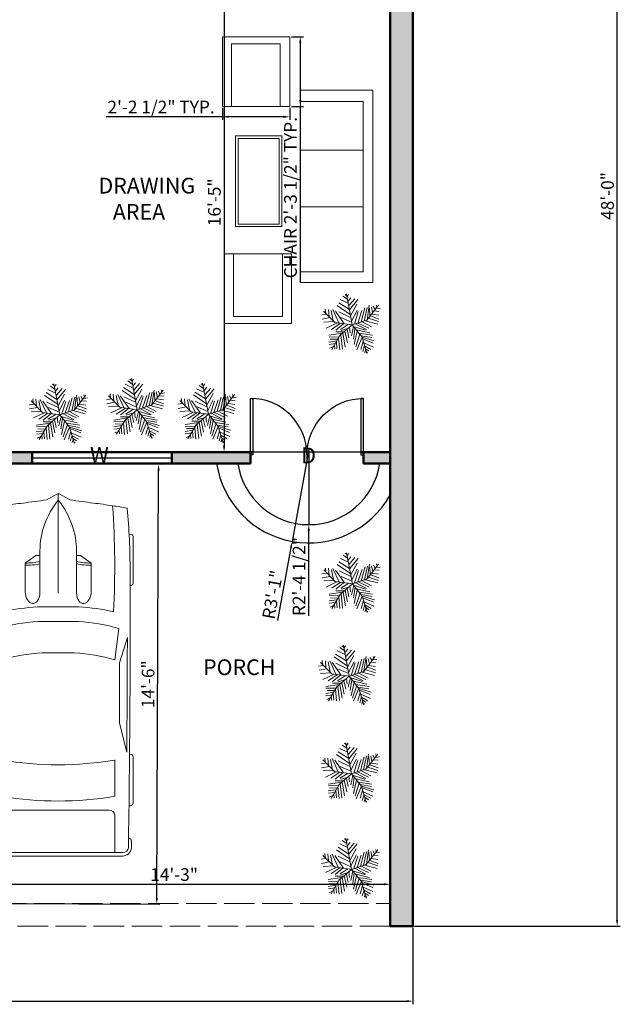
# Model space of a CAD drawing. Units: inches. Extents: x 2227 to 2709, y 1385 to 2029.
# Tile 2 of 4: x 2472 to 2709, y 1385 to 1773. Entities that reach past the tile are written whole.
import ezdxf

# ---------------------------------------------------------------- set-up
doc = ezdxf.new("R2010")
doc.units = ezdxf.units.IN
doc.linetypes.add('ACAD_ISO02W100', pattern=[15, 12, -3])
for name, color, linetype, lineweight in [('A-ANNO-DIMS', 1, 'Continuous', 18), ('A-ANNO-TEXT', 30, 'Continuous', 18), ('A-AREA-IDEN', 30, 'Continuous', 25), ('A-FLOR-STRS', 7, 'Continuous', 25), ('A-FLOR-THRE', 8, 'ACAD_ISO02W100', 18), ('A-FURN', 50, 'Continuous', 18), ('A-SITE-VEHI', 8, 'Continuous', 13), ('A-WALL-PATT', 252, 'Continuous', 13), ('DOOR', 130, 'Continuous', 25), ('TREE', 80, 'Continuous', 13), ('WALL', 160, 'Continuous', 50), ('WIND', 40, 'Continuous', 25)]:
    doc.layers.add(name, color=color, linetype=linetype, lineweight=lineweight)
doc.styles.get("Standard").update_dxf_attribs({"font": 'arial.ttf'})
doc.dimstyles.new('ISO-25', dxfattribs={"dimtxt": 5, "dimasz": 2.5, "dimexe": 1.25, "dimexo": 0.625, "dimtad": 1, "dimdec": 0, "dimlunit": 4, "dimtxsty": 'Standard', "dimcen": 2.5, "dimadec": 0, "dimazin": 0, "dimtfac": 1, "dimtdec": 0, "dimtmove": 0, "dimatfit": 3, "dimfxl": 1, "dimarcsym": 0})

# ---------------------------------------------------------------- blocks, each defined once
blk = doc.blocks.new('*U8')
for p, q in [((21.1, 37.41), (21.1, 36.83)), ((46.55, 38.89), (22.35, 38.89)), ((47.8, 37.39), (47.8, 37.41)), ((87.99, 31.87), (74.76, 35.92)), ((135.45, 37.07), (135.45, 37.41)), ((136.7, 38.89), (160.9, 38.89)), ((162.15, 37.41), (162.15, 36.77)), ((70.03, 31.54), (86.41, 29.35)), ((134.31, 35.6), (119.29, 31.78)), ((186.47, -33.5), (186.47, 33.5)), ((188.4, -32.76), (188.4, 32.76)), ((138.42, 29.35), (157.25, 29.35)), ((164.52, 26.39), (164.52, -26.39)), ((186.47, 29.35), (167.01, 29.35)), ((32.27, 11.63), (36.13, 17.17)), ((36.13, 17.17), (50.94, 17.17)), ((32.12, 9.51), (32.12, 11.15)), ((58.92, -10.77), (58.92, 10.77)), ((66.55, -10.53), (66.55, 10.53)), ((186.47, -10.53), (186.47, 10.53)), ((3.27, 6.13), (0.1, 0.41)), ((29.77, 9.51), (51.68, 9.51)), ((82.74, 8.5), (82.74, -8.5)), ((0, 0), (51.68, 0)), ((0.1, -0.41), (3.27, -6.13)), ((29.77, -9.51), (51.68, -9.51)), ((32.12, -9.51), (32.12, -11.15)), ((32.27, -11.63), (36.13, -17.17)), ((36.13, -17.17), (50.94, -17.17)), ((86.41, -29.35), (70.03, -31.54)), ((157.25, -29.35), (138.42, -29.35)), ((167.01, -29.35), (186.47, -29.35)), ((87.99, -31.87), (74.76, -35.92)), ((134.31, -35.6), (119.29, -31.78)), ((21.1, -37.41), (21.1, -36.83)), ((46.55, -38.89), (22.35, -38.89)), ((47.8, -37.39), (47.8, -37.41)), ((135.45, -37.07), (135.45, -37.41)), ((136.7, -38.89), (160.9, -38.89)), ((162.15, -37.41), (162.15, -36.77))]:
    blk.add_line(p, q)
for centre, major_axis, ratio, start_param, end_param in [((266.03, -27.52), (0, 313.31), 0.842304, 1.367076, 1.39176), ((41.19, -490.86), (0, 528.23), 0.842304, 0.00281, 0.075598), ((22.35, 37.41), (0, -1.48), 0.842304, 3.141593, 4.712389), ((64.48, -10555.62), (0, 10593.03), 0.842304, -0.013397, 0.002797), ((46.55, 37.41), (0, 1.48), 0.842304, -1.570796, 0), ((64.48, -10555.62), (0, -10591.55), 0.842304, 3.133765, 3.140441), ((136.7, 37.41), (0, -1.48), 0.842304, 3.141593, 4.712389), ((160.9, 37.41), (0, 1.48), 0.842304, -1.570796, 0), ((180.63, 35.84), (0, 2.22), 0.842304, -0.013017, 1.249894), ((64.48, -10556.36), (0, 10595.31), 0.842304, -0.013397, -0.013017), ((183.98, 33.5), (0, -2.96), 0.842304, 1.570796, 3.128196), ((183.98, 32.76), (0, -5.25), 0.842304, 1.570796, 3.128196), ((135.29, 5.39), (0, 81.77), 0.842304, 1.245306, 1.50788), ((95.79, -3666.35), (0, -3698.24), 0.842304, 3.134049, 3.144098), ((259.18, -27.52), (0, -305.3), 0.842304, 4.528606, 4.561838), ((37.47, -593.96), (0, -623.33), 0.842304, 3.096046, 3.200911), ((134.4, 5.39), (0, -89.78), 0.842304, 4.449482, 4.652344), ((149.6, 2.8), (0, -79.58), 0.842304, 4.372215, 4.640744), ((17.08, 0), (0, 147.02), 0.842304, 4.511394, 4.913384), ((35.91, 0), (0, 147.02), 0.842304, 4.511394, 4.913384), ((167.01, 26.39), (0, 2.96), 0.842304, 0, 1.570796), ((-204.49, 52.4), (0, -250.96), 0.842304, 1.385369, 1.434372), ((13.04, 17.01), (0, 27.42), 0.842304, 4.435146, 4.718221), ((14.2, 17.01), (0, 27.42), 0.842304, 4.435146, 4.718221), ((50.79, 13.34), (6.34, -0.36), 0.603834, -1.395552, 1.581315), ((32.75, 11.15), (0, 0.74), 0.842304, 0.879714, 1.570796), ((29.77, -46.66), (0, 56.17), 0.842304, 0, 0.590319), ((0.62, 0), (0, -0.74), 0.842304, 4.131459, 5.293319), ((29.77, 46.66), (0, 56.17), 0.842304, 2.551274, 3.141593), ((-204.49, -52.4), (0, 250.96), 0.842304, -1.434372, -1.385369), ((13.04, -17.01), (0, -27.42), 0.842304, 1.564964, 1.848039), ((14.2, -17.01), (0, -27.42), 0.842304, 1.564964, 1.848039), ((149.6, -2.8), (0, -79.58), 0.842304, -1.499151, -1.230623), ((32.75, -11.15), (0, -0.74), 0.842304, 4.712389, 5.403472), ((134.4, -5.39), (0, -89.78), 0.842304, -1.510751, -1.307889), ((135.29, -5.39), (0, -81.77), 0.842304, -1.50788, -1.245306), ((259.18, 27.52), (0, 305.3), 0.842304, 1.721348, 1.754579), ((266.03, 27.52), (0, 313.31), 0.842304, 1.749832, 1.774517), ((37.47, 593.96), (0, -623.33), 0.842304, -0.059319, 0.045547), ((167.01, -26.39), (0, -2.96), 0.842304, 4.712389, 6.283185), ((64.48, 10555.62), (0, -10591.55), 0.842304, 0.001152, 0.007828), ((95.79, 3666.35), (0, -3698.24), 0.842304, -0.002505, 0.007544), ((183.98, -33.5), (0, 2.96), 0.842304, 3.15499, 4.712389), ((183.98, -32.76), (0, -5.25), 0.842304, 0.013397, 1.570796), ((41.19, 490.86), (0, -528.23), 0.842304, -0.075598, -0.00281), ((22.35, -37.41), (0, 1.48), 0.842304, 1.570796, 3.141593), ((64.48, 10555.62), (0, 10593.03), 0.842304, 3.138796, 3.15499), ((46.55, -37.41), (0, -1.48), 0.842304, 0, 1.570796), ((136.7, -37.41), (0, -1.48), 0.842304, -1.570796, 0), ((160.9, -37.41), (0, 1.48), 0.842304, 3.141593, 4.712389), ((180.63, -35.84), (0, -2.22), 0.842304, -1.249894, 0.013017), ((64.48, 10556.36), (0, 10595.31), 0.842304, 3.15461, 3.15499)]:
    blk.add_ellipse(centre, major_axis=major_axis, ratio=ratio, start_param=start_param, end_param=end_param)
at = {"extrusion": (0, 0, -1)}
blk.add_ellipse((50.79, -13.34), major_axis=(6.34, 0.36), ratio=0.603834, start_param=-1.395552, end_param=1.581315, dxfattribs=at)
blk = doc.blocks.new('*U2')
for p, q in [((0, 0), (0, -6)), ((40, 0), (40, -6))]:
    blk.add_line(p, q)
blk.add_lwpolyline([(0, 0), (0, 40), (1.75, 40), (1.75, 0)], close=True)
blk.add_arc((0, 0), 40, 0, 90)
blk = doc.blocks.new('*U6')
for p, q in [((-10.186, 53.64), (-13.084, 55.962)), ((0, 0), (-10.5, 57)), ((-9.099, 51.782), (-6.563, 55.962)), ((-5.114, 28.097), (-24.676, 40.636)), ((-7.288, 39.707), (-21.778, 46.673)), ((-8.737, 47.138), (-17.069, 52.711)), ((-7.65, 43.423), (-2.578, 49.46)), ((-5.839, 35.992), (4.667, 48.067)), ((-5.114, 27.632), (10.463, 46.673)), ((-2.941, 16.486), (8.652, 37.85)), ((44.153, 36.456), (45.239, 32.741)), ((-47.498, 19.737), (-55.83, 18.344)), ((-31.5, 4.5), (-52.5, 25.5)), ((-48.585, 21.131), (-49.309, 29.026)), ((-43.513, 28.561), (-42.427, 15.558)), ((-38.442, 26.239), (-34.819, 7.663)), ((-35.544, 28.097), (-24.314, 3.947)), ((-14.533, 2.09), (-30.834, 25.31)), ((-3.665, 19.273), (-27.574, 35.527)), ((-24.314, 23.917), (-2.941, 13.7)), ((-1.129, 6.734), (9.014, 26.704)), ((3.942, 1.625), (11.187, 24.381)), ((10.101, 3.483), (17.708, 26.239)), ((16.259, 5.805), (23.142, 31.348)), ((22.055, 7.198), (27.489, 32.277)), ((27, 9), (48, 36)), ((27.127, 9.056), (31.112, 35.992)), ((31.836, 30.883), (32.561, 16.486)), ((35.096, 32.741), (37.27, 22.524)), ((36.183, 19.737), (48.137, 17.88)), ((38.719, 34.134), (41.979, 28.561)), ((40.53, 25.775), (48.862, 24.846)), ((43.791, 29.954), (51.036, 30.883)), ((-40.615, 13.7), (-55.105, 10.913)), ((-33.37, 6.269), (-52.207, 5.34)), ((-28.299, 3.483), (-47.86, -5.805)), ((-21.416, 3.018), (-38.079, -8.128)), ((0, 0), (-31.5, 4.5)), ((-15.982, 2.09), (-30.11, -9.521)), ((0, 0), (-22.5, -19.5)), ((-6.563, 1.161), (-21.416, -8.128)), ((-20.691, 13.7), (-1.129, 4.876)), ((0, 0), (27, 9)), ((0, 0), (18, -22.5)), ((6.478, 1.625), (26.04, -8.592)), ((11.187, 3.483), (30.749, -5.805)), ((18.07, 5.805), (35.096, -3.483)), ((24.229, 7.663), (46.688, 1.625)), ((29.662, 12.307), (48.137, 6.269)), ((33.285, 16.486), (48.862, 10.913)), ((-17.431, -15.094), (-42.789, -18.809)), ((-15.257, -12.772), (-30.11, -12.772)), ((-6.563, -5.805), (-19.967, -9.985)), ((-17.069, -15.094), (-12.721, -40.172)), ((-13.446, -11.378), (-8.737, -32.741)), ((-9.461, -8.592), (-6.201, -23.453)), ((-4.752, -3.483), (-3.665, -14.629)), ((2.493, -3.019), (-1.491, -20.202)), ((1.769, -2.555), (24.229, -9.521)), ((5.029, -6.27), (2.131, -25.775)), ((9.014, -11.378), (3.58, -35.992)), ((14.085, -16.951), (6.478, -40.172)), ((7.565, -9.056), (32.198, -14.629)), ((12.274, -15.094), (36.907, -18.809)), ((-28.299, -29.026), (-42.789, -31.348)), ((-24.314, -21.596), (-42.427, -22.06)), ((-30.834, -34.135), (-42.427, -35.528)), ((-26.849, -26.24), (-40.253, -25.775)), ((-22.5, -19.5), (-37.5, -45)), ((-29.023, -30.884), (-27.936, -43.887)), ((-25.038, -23.918), (-22.865, -45.281)), ((-20.691, -18.345), (-17.793, -44.352)), ((18.07, -22.524), (8.289, -45.745)), ((20.244, -30.419), (15.897, -44.816)), ((16.259, -19.738), (36.183, -22.989)), ((18, -22.5), (27, -52.5)), ((18.433, -22.524), (40.53, -29.026)), ((19.157, -25.311), (38.719, -33.206)), ((21.331, -32.741), (39.081, -40.636)), ((-34.457, -39.708), (-40.978, -42.494)), ((-32.646, -36.921), (-31.921, -44.352)), ((22.78, -37.85), (19.519, -48.532)), ((22.78, -38.314), (34.372, -44.816)), ((24.591, -45.745), (23.142, -50.854)), ((24.591, -43.423), (30.749, -47.603)), ((26.764, -49.925), (28.213, -50.854))]:
    blk.add_line(p, q)
blk = doc.blocks.new('*D27')
at = {"layer": 'A-ANNO-DIMS', "color": 0, "lineweight": -2, "transparency": 16777216}
for p, q in [((2447.21, 1424.96), (2447.21, 1433.13)), ((2617.71, 1424.96), (2617.71, 1433.13)), ((2449.71, 1431.88), (2615.21, 1431.88))]:
    blk.add_line(p, q, dxfattribs=at)
at = {"layer": 'A-ANNO-DIMS', "color": 0, "lineweight": 100, "transparency": 16777216}
for points in [[(2449.71, 1432.3), (2449.71, 1431.46), (2447.21, 1431.88)], [(2615.21, 1432.3), (2615.21, 1431.46), (2617.71, 1431.88)]]:
    blk.add_solid(points, dxfattribs=at)
at = {"layer": 'Defpoints', "color": 0, "lineweight": 100, "transparency": 16777216}
for p in [(2617.71, 1431.88), (2447.21, 1424.33), (2617.71, 1424.33)]:
    blk.add_point(p, dxfattribs=at)
at = {"layer": 'A-ANNO-DIMS', "color": 0, "transparency": 16777216, "insert": (2532.46, 1435.06), "char_height": 5, "attachment_point": 5}
blk.add_mtext('14\'-3"', dxfattribs=at)
blk = doc.blocks.new('*D28')
at = {"layer": 'A-ANNO-DIMS', "color": 0, "lineweight": -2, "transparency": 16777216}
for p, q in [((2448.57, 1597.83), (2527.6, 1597.5)), ((2525.63, 1426.5), (2526.34, 1595)), ((2447.84, 1424.33), (2526.87, 1424))]:
    blk.add_line(p, q, dxfattribs=at)
at = {"layer": 'A-ANNO-DIMS', "color": 0, "lineweight": 100, "transparency": 16777216}
for points in [[(2525.92, 1595), (2526.75, 1595), (2526.35, 1597.5)], [(2525.21, 1426.5), (2526.04, 1426.5), (2525.62, 1424)]]:
    blk.add_solid(points, dxfattribs=at)
at = {"layer": 'Defpoints', "color": 0, "lineweight": 100, "transparency": 16777216}
for p in [(2447.95, 1597.83), (2526.35, 1597.5), (2447.21, 1424.33)]:
    blk.add_point(p, dxfattribs=at)
at = {"layer": 'A-ANNO-DIMS', "color": 0, "transparency": 16777216, "insert": (2522.8, 1510.77), "char_height": 5, "attachment_point": 5, "rotation": 89.7584}
blk.add_mtext('14\'-6"', dxfattribs=at)
blk = doc.blocks.new('*D30')
at = {"layer": 'A-ANNO-DIMS', "color": 0, "lineweight": -2, "transparency": 16777216}
for p, q in [((2617.09, 1799.33), (2550.92, 1799.33)), ((2552.17, 1796.83), (2552.17, 1604.83)), ((2617.09, 1602.33), (2550.92, 1602.33))]:
    blk.add_line(p, q, dxfattribs=at)
at = {"layer": 'A-ANNO-DIMS', "color": 0, "lineweight": 100, "transparency": 16777216}
for points in [[(2551.76, 1796.83), (2552.59, 1796.83), (2552.17, 1799.33)], [(2551.76, 1604.83), (2552.59, 1604.83), (2552.17, 1602.33)]]:
    blk.add_solid(points, dxfattribs=at)
at = {"layer": 'Defpoints', "color": 0, "lineweight": 100, "transparency": 16777216}
for p in [(2617.71, 1799.33), (2552.17, 1602.33), (2617.71, 1602.33)]:
    blk.add_point(p, dxfattribs=at)
at = {"layer": 'A-ANNO-DIMS', "color": 0, "transparency": 16777216, "insert": (2548.99, 1700.83), "char_height": 5, "attachment_point": 5, "rotation": 90}
blk.add_mtext('16\'-5"', dxfattribs=at)
blk = doc.blocks.new('ARMCHAIR')
for p, q in [((0, 0), (-3.76, 0)), ((-3.76, 0), (-3.76, -27.46)), ((0, 0), (0, -24.72)), ((19.25, 0), (22.81, 0)), ((22.81, 0), (22.81, -27.46)), ((22.81, -27.46), (-3.76, -27.46))]:
    blk.add_line(p, q)
blk.add_lwpolyline([(0, -24.72), (19.25, -24.72), (19.25, 0), (0, 0)])
blk = doc.blocks.new('*D43')
at = {"layer": 'A-ANNO-DIMS', "color": 0, "lineweight": -2, "transparency": 16777216}
for p, q in [((2578.74, 1766.14), (2583.48, 1766.14)), ((2582.23, 1763.64), (2582.23, 1741.17)), ((2578.74, 1738.67), (2583.48, 1738.67)), ((2582.23, 1738.67), (2582.23, 1669.18))]:
    blk.add_line(p, q, dxfattribs=at)
at = {"layer": 'A-ANNO-DIMS', "color": 0, "lineweight": 100, "transparency": 16777216}
for points in [[(2581.81, 1763.64), (2582.65, 1763.64), (2582.23, 1766.14)], [(2581.81, 1741.17), (2582.65, 1741.17), (2582.23, 1738.67)]]:
    blk.add_solid(points, dxfattribs=at)
at = {"layer": 'Defpoints', "color": 0, "lineweight": 100, "transparency": 16777216}
for p in [(2578.11, 1766.14), (2578.11, 1738.67), (2582.23, 1738.67)]:
    blk.add_point(p, dxfattribs=at)
at = {"layer": 'A-ANNO-DIMS', "color": 0, "transparency": 16777216, "insert": (2579.02, 1702.67), "char_height": 5, "attachment_point": 5, "rotation": 90}
blk.add_mtext('CHAIR 2\'-3 1/2" TYP.', dxfattribs=at)
blk = doc.blocks.new('*D44')
at = {"layer": 'A-ANNO-DIMS', "color": 0, "lineweight": -2, "transparency": 16777216}
for p, q in [((2551.54, 1738.05), (2551.54, 1733.3)), ((2578.11, 1738.05), (2578.11, 1733.3)), ((2551.54, 1734.55), (2505.58, 1734.55)), ((2575.61, 1734.55), (2554.04, 1734.55))]:
    blk.add_line(p, q, dxfattribs=at)
at = {"layer": 'A-ANNO-DIMS', "color": 0, "lineweight": 100, "transparency": 16777216}
for points in [[(2554.04, 1734.97), (2554.04, 1734.13), (2551.54, 1734.55)], [(2575.61, 1734.97), (2575.61, 1734.13), (2578.11, 1734.55)]]:
    blk.add_solid(points, dxfattribs=at)
at = {"layer": 'Defpoints', "color": 0, "lineweight": 100, "transparency": 16777216}
for p in [(2551.54, 1738.67), (2578.11, 1738.67), (2551.54, 1734.55)]:
    blk.add_point(p, dxfattribs=at)
at = {"layer": 'A-ANNO-DIMS', "color": 0, "transparency": 16777216, "insert": (2527.31, 1737.76), "char_height": 5, "attachment_point": 5}
blk.add_mtext('2\'-2 1/2" TYP.', dxfattribs=at)
blk = doc.blocks.new('*D47')
at = {"layer": 'A-ANNO-DIMS', "color": 0, "lineweight": -2, "transparency": 16777216}
for p, q in [((2290.71, 1414.71), (2290.71, 1384.53)), ((2626.71, 1414.71), (2626.71, 1384.53)), ((2293.21, 1385.78), (2624.21, 1385.78))]:
    blk.add_line(p, q, dxfattribs=at)
at = {"layer": 'A-ANNO-DIMS', "color": 0, "lineweight": 100, "transparency": 16777216}
for points in [[(2293.21, 1386.2), (2293.21, 1385.37), (2290.71, 1385.78)], [(2624.21, 1386.2), (2624.21, 1385.37), (2626.71, 1385.78)]]:
    blk.add_solid(points, dxfattribs=at)
at = {"layer": 'Defpoints', "color": 0, "lineweight": 100, "transparency": 16777216}
for p in [(2290.71, 1415.33), (2626.71, 1415.33), (2626.71, 1385.78)]:
    blk.add_point(p, dxfattribs=at)
at = {"layer": 'A-ANNO-DIMS', "color": 0, "transparency": 16777216, "insert": (2458.71, 1388.96), "char_height": 5, "attachment_point": 5}
blk.add_mtext('28\'-0"', dxfattribs=at)
blk = doc.blocks.new('*D48')
at = {"layer": 'A-ANNO-DIMS', "color": 0, "lineweight": -2, "transparency": 16777216}
for p, q in [((2627.34, 1991.33), (2708.51, 1991.33)), ((2707.26, 1417.83), (2707.26, 1988.83)), ((2627.34, 1415.33), (2708.51, 1415.33))]:
    blk.add_line(p, q, dxfattribs=at)
at = {"layer": 'A-ANNO-DIMS', "color": 0, "lineweight": 100, "transparency": 16777216}
for points in [[(2706.85, 1988.83), (2707.68, 1988.83), (2707.26, 1991.33)], [(2706.85, 1417.83), (2707.68, 1417.83), (2707.26, 1415.33)]]:
    blk.add_solid(points, dxfattribs=at)
at = {"layer": 'Defpoints', "color": 0, "lineweight": 100, "transparency": 16777216}
for p in [(2626.71, 1991.33), (2707.26, 1991.33), (2626.71, 1415.33)]:
    blk.add_point(p, dxfattribs=at)
at = {"layer": 'A-ANNO-DIMS', "color": 0, "transparency": 16777216, "insert": (2704.09, 1703.33), "char_height": 5, "attachment_point": 5, "rotation": 90}
blk.add_mtext('48\'-0"', dxfattribs=at)
blk = doc.blocks.new('*D51')
at = {"layer": 'A-ANNO-DIMS', "color": 0, "lineweight": -2, "transparency": 16777216}
for p, q in [((2585.59, 1603.29), (2579.02, 1567.11)), ((2573.36, 1535.9), (2578.58, 1564.65))]:
    blk.add_line(p, q, dxfattribs=at)
at = {"layer": 'A-ANNO-DIMS', "color": 0, "lineweight": 100, "transparency": 16777216}
blk.add_solid([(2578.17, 1564.73), (2578.99, 1564.58), (2579.02, 1567.11)], dxfattribs=at)
at = {"layer": 'Defpoints', "color": 0, "lineweight": 100, "transparency": 16777216}
for p in [(2585.59, 1603.29), (2579.02, 1567.11)]:
    blk.add_point(p, dxfattribs=at)
at = {"layer": 'A-ANNO-DIMS', "color": 0, "transparency": 16777216, "insert": (2571.96, 1545.97), "char_height": 5, "attachment_point": 5, "rotation": 79.7207}
blk.add_mtext('R3\'-1"', dxfattribs=at)
blk = doc.blocks.new('*D52')
at = {"layer": 'A-ANNO-DIMS', "color": 0, "lineweight": -2, "transparency": 16777216}
for p, q in [((2585.59, 1602.04), (2585.58, 1573.71)), ((2585.58, 1537.73), (2585.58, 1571.21))]:
    blk.add_line(p, q, dxfattribs=at)
at = {"layer": 'A-ANNO-DIMS', "color": 0, "lineweight": 100, "transparency": 16777216}
blk.add_solid([(2585.17, 1571.21), (2586, 1571.21), (2585.58, 1573.71)], dxfattribs=at)
at = {"layer": 'Defpoints', "color": 0, "lineweight": 100, "transparency": 16777216}
for p in [(2585.59, 1602.04), (2585.58, 1573.71)]:
    blk.add_point(p, dxfattribs=at)
at = {"layer": 'A-ANNO-DIMS', "color": 0, "transparency": 16777216, "insert": (2582.37, 1553.22), "char_height": 5, "attachment_point": 5, "rotation": 89.9996}
blk.add_mtext('R2\'-4 1/2"', dxfattribs=at)

msp = doc.modelspace()

# ---------------------------------------------------------------- hatches: boundary and pattern name
at = {"layer": 'A-WALL-PATT'}
h = msp.add_hatch(color=256, dxfattribs=at)
h.dxf.hatch_style = 1
h.paths.add_polyline_path([(2538.21, 1991.33), (2290.71, 1991.33), (2290.71, 1982.33), (2299.71, 1982.33), (2538.21, 1982.33)])
h.paths.add_polyline_path([(2299.71, 1982.33), (2290.71, 1982.33), (2290.71, 1424.33), (2299.71, 1424.33)])
h.paths.add_polyline_path([(2347.13, 1424.33), (2290.71, 1424.33), (2290.71, 1415.33), (2347.13, 1415.33)])
h.paths.add_polyline_path([(2447.21, 1424.33), (2402.93, 1424.33), (2402.93, 1415.33), (2447.21, 1415.33)])
h.paths.add_polyline_path([(2447.21, 1597.83), (2442.71, 1597.83), (2442.71, 1424.33), (2447.21, 1424.33)])
h.paths.add_polyline_path([(2396.41, 1528.83), (2299.71, 1528.83), (2299.71, 1524.33), (2396.41, 1524.33)])
h.paths.add_polyline_path([(2442.71, 1528.83), (2436.41, 1528.83), (2436.41, 1524.33), (2442.71, 1524.33)])
h.paths.add_polyline_path([(2345.64, 1667.33), (2299.71, 1667.33), (2299.71, 1662.83), (2345.64, 1662.83)])
h.paths.add_polyline_path([(2447.21, 1747.77), (2442.71, 1747.77), (2442.71, 1662.83), (2447.21, 1662.83)])
h.paths.add_polyline_path([(2442.71, 1667.33), (2401.29, 1667.33), (2401.29, 1662.83), (2442.71, 1662.83)])
h.paths.add_polyline_path([(2447.21, 1803.83), (2299.71, 1803.83), (2299.71, 1799.33), (2447.21, 1799.33)])
h.paths.add_polyline_path([(2447.21, 1799.33), (2442.71, 1799.33), (2442.71, 1787.77), (2447.21, 1787.77)])
h.paths.add_polyline_path([(2394.45, 1851.83), (2389.95, 1851.83), (2389.95, 1803.83), (2394.45, 1803.83)])
h.paths.add_polyline_path([(2327.17, 1851.83), (2322.67, 1851.83), (2322.67, 1840.2), (2327.17, 1840.2)])
h.paths.add_polyline_path([(2327.17, 1815.42), (2322.67, 1815.42), (2322.67, 1803.83), (2327.17, 1803.83)])
h.paths.add_polyline_path([(2397.41, 1856.33), (2299.71, 1856.33), (2299.71, 1851.83), (2397.41, 1851.83)])
h.paths.add_polyline_path([(2447.21, 1856.33), (2437.41, 1856.33), (2437.41, 1851.83), (2447.21, 1851.83)])
h.paths.add_polyline_path([(2447.21, 1934.33), (2442.71, 1934.33), (2442.71, 1856.33), (2447.21, 1856.33)])
h.paths.add_polyline_path([(2459.62, 1856.33), (2447.21, 1856.33), (2447.21, 1851.83), (2459.62, 1851.83)])
h.paths.add_polyline_path([(2498.21, 1856.33), (2494.53, 1856.33), (2494.53, 1851.83), (2498.21, 1851.83)])
h.paths.add_polyline_path([(2462.23, 1934.33), (2447.21, 1934.33), (2447.21, 1929.83), (2462.23, 1929.83)])
h.paths.add_polyline_path([(2507.32, 1934.33), (2483.3, 1934.33), (2483.3, 1929.83), (2507.32, 1929.83)])
h.paths.add_polyline_path([(2542.71, 1947.66), (2538.21, 1947.66), (2538.21, 1934.33), (2542.71, 1934.33)])
h.paths.add_polyline_path([(2544.78, 1934.33), (2536.35, 1934.33), (2536.35, 1929.83), (2544.78, 1929.83)])
h.paths.add_polyline_path([(2542.71, 1982.33), (2538.21, 1982.33), (2538.21, 1971.57), (2542.71, 1971.57)])
h.paths.add_polyline_path([(2346.6, 1815.57), (2382.82, 1815.57), (2382.82, 1838.66), (2346.6, 1838.66)], flags=9)
h.paths.add_polyline_path([(2457.86, 1902.08), (2494.08, 1902.08), (2494.08, 1925.17), (2457.86, 1925.17)], flags=9)
h.paths.add_polyline_path([(2500.39, 1690.49), (2545.31, 1690.49), (2545.31, 1713.58), (2500.39, 1713.58)], flags=9)
h.paths.add_polyline_path([(2528.08, 1476.92), (2562.42, 1476.92), (2562.42, 1489.69), (2528.08, 1489.69)], flags=9)
h.paths.add_polyline_path([(2349.07, 1476.93), (2390.15, 1476.93), (2390.15, 1489.69), (2349.07, 1489.69)], flags=9)
h.paths.add_polyline_path([(2347.99, 1586.39), (2381.37, 1586.39), (2381.37, 1609.48), (2347.99, 1609.48)], flags=9)
h.paths.add_polyline_path([(2328.07, 1742.46), (2375.88, 1742.46), (2375.88, 1755.23), (2328.07, 1755.23)], flags=9)
h.paths.add_polyline_path([(2556.42, 1893.75), (2604.23, 1893.75), (2604.23, 1906.51), (2556.42, 1906.51)], flags=9)
h.paths.add_polyline_path([(2323.02, 1893.88), (2370.83, 1893.88), (2370.83, 1906.64), (2323.02, 1906.64)], flags=9)
h.paths.add_polyline_path([(2562.19, 1958.77), (2598.41, 1958.77), (2598.41, 1981.86), (2562.19, 1981.86)], flags=9)
h.paths.add_polyline_path([(2482.23, 1953.14), (2507.92, 1953.14), (2507.92, 1965.9), (2482.23, 1965.9)], flags=9)
h = msp.add_hatch(color=256, dxfattribs=at)
h.dxf.hatch_style = 1
h.paths.add_polyline_path([(2617.71, 1991.33), (2538.21, 1991.33), (2538.21, 1982.33), (2617.71, 1982.33)])
h.paths.add_polyline_path([(2626.71, 1991.33), (2617.71, 1991.33), (2617.71, 1982.33), (2617.71, 1415.33), (2626.71, 1415.33)])
h.paths.add_polyline_path([(2617.71, 1934.33), (2577.48, 1934.33), (2577.48, 1929.83), (2617.71, 1929.83)])
h.paths.add_polyline_path([(2502.71, 1929.83), (2498.21, 1929.83), (2498.21, 1803.83), (2502.71, 1803.83)])
h.paths.add_polyline_path([(2617.71, 1803.83), (2547.01, 1803.83), (2547.01, 1799.33), (2617.71, 1799.33)])
h.paths.add_polyline_path([(2507.01, 1803.83), (2498.21, 1803.83), (2498.21, 1799.33), (2507.01, 1799.33)])
h.paths.add_polyline_path([(2617.71, 1602.33), (2607.17, 1602.33), (2607.17, 1601.18), (2607.17, 1597.83), (2617.71, 1597.83)])
h = msp.add_hatch(color=256, dxfattribs=at)
h.dxf.hatch_style = 1
h.paths.add_polyline_path([(2476.5, 1602.33), (2447.21, 1602.33), (2447.21, 1597.83), (2476.5, 1597.83)])
h.paths.add_polyline_path([(2447.21, 1602.33), (2442.71, 1602.33), (2442.71, 1597.83), (2447.21, 1597.83)])
h = msp.add_hatch(color=256, dxfattribs=at)
h.dxf.hatch_style = 1
h.paths.add_polyline_path([(2562.56, 1602.33), (2531.5, 1602.33), (2531.5, 1597.83), (2562.56, 1597.83), (2562.56, 1601.18)])

# ---------------------------------------------------------------- linework, layer by layer
at = {"layer": 'A-FLOR-STRS'}
for centre, radius, end in [((2585.59, 1603.29), 36.77, 330.9045), ((2585.59, 1602.04), 28.33, 351.4629)]:
    msp.add_arc(centre, radius, 188.5371, end, dxfattribs=at)
at = {"layer": 'A-FLOR-THRE'}
msp.add_lwpolyline([(2617.71, 1415.33), (2447.21, 1415.33), (2447.21, 1424.33), (2617.71, 1424.33)], close=True, dxfattribs=at)
at = {"layer": 'A-FURN'}
for p, q in [((2582.29, 1740.64), (2582.29, 1745)), ((2582.29, 1745), (2610.85, 1745)), ((2610.85, 1745), (2610.85, 1669.26)), ((2582.29, 1721.39), (2607.01, 1721.39)), ((2582.29, 1699), (2607.01, 1699)), ((2582.29, 1669.26), (2582.29, 1673.4)), ((2610.85, 1669.26), (2582.29, 1669.26))]:
    msp.add_line(p, q, dxfattribs=at)
for points in [[(2607.01, 1740.64), (2582.29, 1740.64), (2582.29, 1673.4), (2607.01, 1673.4)], [(2556.69, 1726.99), (2574.94, 1726.99), (2574.94, 1691.24), (2556.69, 1691.24)], [(2557.69, 1725.99), (2573.94, 1725.99), (2573.94, 1692.24), (2557.69, 1692.24)]]:
    msp.add_lwpolyline(points, close=True, dxfattribs=at)
at = {"layer": 'WALL'}
for p, q in [((2626.71, 1991.33), (2626.71, 1415.33)), ((2617.71, 1799.33), (2617.71, 1602.33)), ((2563.54, 1602.33), (2447.21, 1602.33)), ((2584.9, 1602.33), (2584.84, 1602.33)), ((2617.71, 1602.33), (2606.2, 1602.33)), ((2562.56, 1597.83), (2447.21, 1597.83)), ((2617.71, 1597.83), (2607.17, 1597.83)), ((2617.71, 1424.33), (2617.71, 1415.33)), ((2626.71, 1415.33), (2617.71, 1415.33))]:
    msp.add_line(p, q, dxfattribs=at)
for points in [[(2447.21, 1415.33), (2290.71, 1415.33), (2290.71, 1991.33), (2626.71, 1991.33), (2626.71, 1415.33), (2617.71, 1415.33)], [(2447.21, 1424.33), (2299.71, 1424.33), (2299.71, 1982.33), (2617.71, 1982.33), (2617.71, 1424.33)]]:
    msp.add_lwpolyline(points, dxfattribs=at)
for points in [[(2617.71, 1991.33), (2626.71, 1991.33), (2626.71, 1415.33), (2617.71, 1415.33)], [(2476.5, 1597.83), (2442.71, 1597.83), (2442.71, 1602.33), (2476.5, 1602.33)], [(2531.5, 1602.33), (2562.56, 1602.33), (2562.56, 1597.83), (2531.5, 1597.83)], [(2607.17, 1597.83), (2617.71, 1597.83), (2617.71, 1602.33), (2607.17, 1602.33)]]:
    msp.add_lwpolyline(points, close=True, dxfattribs=at)
at = {"layer": 'WIND'}
msp.add_line((2476.5, 1600.08), (2531.5, 1600.08), dxfattribs=at)
msp.add_lwpolyline([(2476.5, 1597.83), (2531.5, 1597.83), (2531.5, 1602.33), (2476.5, 1602.33)], close=True, dxfattribs=at)

# ---------------------------------------------------------------- block references
at = {"layer": 'A-FURN', "rotation": 180}
msp.add_blockref('ARMCHAIR', (2574.35, 1738.67), dxfattribs=at)
at = {"layer": 'A-FURN'}
msp.add_blockref('ARMCHAIR', (2555.93, 1680.46), dxfattribs=at)
at = {"layer": 'A-SITE-VEHI', "xscale": 0.7592338351004116, "yscale": 0.7592338351004116, "zscale": 0.7592338351004116, "rotation": 270}
msp.add_blockref('*U8', (2486.73, 1585.98), dxfattribs=at)
at = {"layer": 'DOOR', "yscale": 0.5576621142941873, "zscale": 0.5576621142941873}
for p, xscale in [((2562.56, 1601.18), 0.5576621142941873), ((2607.17, 1601.18), -0.5576621142941873)]:
    msp.add_blockref('*U2', p, dxfattribs=dict(at, xscale=xscale))
at = {"layer": 'TREE', "xscale": 0.2153773147918839, "yscale": 0.2153773147918839, "zscale": 0.2153773147918839}
for p in [(2602.72, 1652.46), (2517.84, 1619.02), (2487.3, 1617.02), (2545.98, 1617.22), (2602.79, 1550.35), (2601.5, 1513.91), (2602.48, 1475.42), (2602.48, 1437.76)]:
    msp.add_blockref('*U6', p, dxfattribs=at)

# ---------------------------------------------------------------- texts
at = {"layer": 'A-ANNO-TEXT', "char_height": 6.19, "attachment_point": 1}
for s, insert in [('W', (2499.26, 1604.34)), ('D', (2582.64, 1604.14))]:
    msp.add_mtext_dynamic_manual_height_columns(s, width=156.7329, gutter_width=30.97, heights=[0], dxfattribs=dict(at, insert=insert))
at = {"layer": 'A-AREA-IDEN', "char_height": 6.194, "attachment_point": 1}
for s, insert in [('DRAWING \\P   AREA', (2502.61, 1710.5)), ('PORCH', (2543.88, 1520.58))]:
    msp.add_mtext_dynamic_manual_height_columns(s, width=156.7329, gutter_width=30.97, heights=[0], dxfattribs=dict(at, insert=insert))

# ---------------------------------------------------------------- dimensions: what is measured, and where the dimension line sits
at = {"layer": 'A-ANNO-DIMS'}
for base, p1, p2, override, picture, middle in [((2707.26, 1991.33), (2626.71, 1415.33), (2626.71, 1991.33), {"dimdec": 1, "dimlfac": 1, "dimrnd": 0, "dimzin": 1, "dimdsep": 46, "dimlunit": 4, "dimfrac": 2}, '*D48', (2704.09, 1703.33)), ((2552.17, 1602.33), (2617.71, 1799.33), (2617.71, 1602.33), {"dimclrd": 0, "dimclre": 0, "dimclrt": 0}, '*D30', (2548.99, 1700.83))]:
    dim = msp.add_linear_dim(base=base, p1=p1, p2=p2, angle=90, dimstyle='ISO-25', override=override, dxfattribs=at)
    dim.commit()
    dim.dimension.update_dxf_attribs({"geometry": picture, "text_midpoint": middle})
for base, p1, p2, angle, text, picture, middle in [((2582.23, 1738.67), (2578.11, 1766.14), (2578.11, 1738.67), 270, 'CHAIR <> TYP.', '*D43', (2579.02, 1702.67)), ((2551.54, 1734.55), (2578.11, 1738.67), (2551.54, 1738.67), 180, '<> TYP.', '*D44', (2527.31, 1737.76))]:
    dim = msp.add_linear_dim(base=base, p1=p1, p2=p2, angle=angle, text=text, dimstyle='ISO-25', override={"dimdec": 1, "dimlfac": 1, "dimrnd": 0, "dimzin": 1, "dimdsep": 46, "dimlunit": 4, "dimfrac": 2}, dxfattribs=at)
    dim.commit()
    dim.dimension.update_dxf_attribs({"geometry": picture, "text_midpoint": middle})
dim = msp.add_radius_dim(center=(2585.59, 1603.29), mpoint=(2579.02, 1567.11), dimstyle='ISO-25', override={"dimdec": 1, "dimlfac": 1, "dimrnd": 0, "dimzin": 1, "dimdsep": 46, "dimlunit": 4, "dimfrac": 2}, dxfattribs=at)
dim.commit()
dim.dimension.update_dxf_attribs({"geometry": '*D51', "text_midpoint": (2575.09, 1545.41), "dimtype": 164})
dim = msp.add_radius_dim(center=(2585.59, 1602.04), mpoint=(2585.59, 1573.71), dimstyle='ISO-25', override={"dimdec": 1, "dimlfac": 1, "dimrnd": 0, "dimzin": 1, "dimdsep": 46, "dimlunit": 4, "dimfrac": 2}, dxfattribs=at)
dim.commit()
dim.dimension.update_dxf_attribs({"geometry": '*D52', "text_midpoint": (2582.37, 1553.22)})
dim = msp.add_aligned_dim(p1=(2447.21, 1424.33), p2=(2447.95, 1597.83), distance=-78.4, dimstyle='ISO-25', override={"dimclrd": 0, "dimclre": 0, "dimclrt": 0}, dxfattribs=at)
dim.commit()
dim.dimension.update_dxf_attribs({"geometry": '*D28', "text_midpoint": (2522.8, 1510.77)})
for base, p1, p2, override, picture, middle in [((2617.71377381, 1431.88045434), (2447.21377381, 1424.33305883), (2617.71377381, 1424.33305883), {"dimclrd": 0, "dimclre": 0, "dimclrt": 0}, '*D27', (2532.46377381, 1435.0600246)), ((2626.71, 1385.78), (2290.71, 1415.33), (2626.71, 1415.33), {"dimdec": 1, "dimlfac": 1, "dimrnd": 0, "dimzin": 1, "dimdsep": 46, "dimlunit": 4, "dimfrac": 2}, '*D47', (2458.71, 1388.96))]:
    dim = msp.add_linear_dim(base=base, p1=p1, p2=p2, dimstyle='ISO-25', override=override, dxfattribs=at)
    dim.commit()
    dim.dimension.update_dxf_attribs({"geometry": picture, "text_midpoint": middle})

doc.saveas('drawing.dxf')
